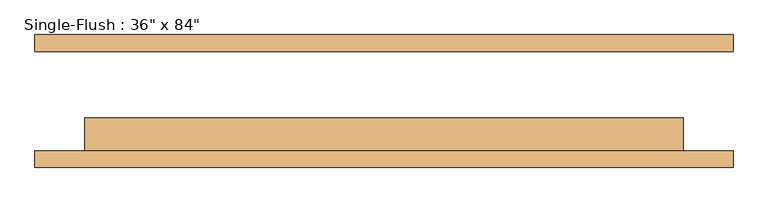
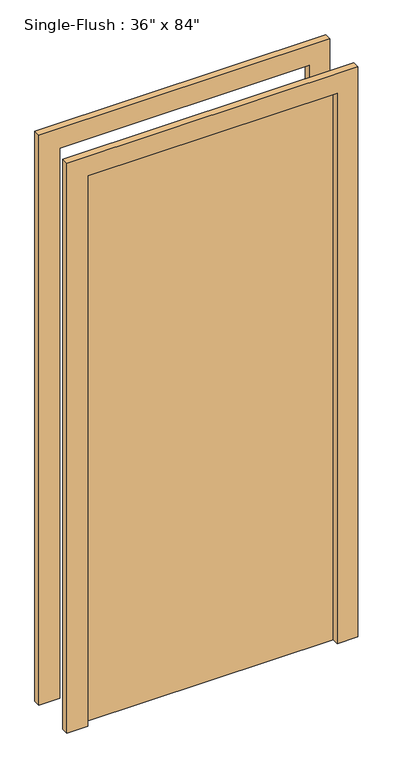
"""IFC4 building model written with IfcOpenShell, lengths in millimetres: door geometry."""

from ifc_helpers import new_model, si_unit, frame, origin, origin_with_axes, place, context, project, spatial, polyline, outline, extrude, source, transform, mapped, element, save


def door_686f89d2(model_context):
    return source(origin(), model_context, "Body", "SweptSolid", [
        extrude(outline(polyline([(2209.8, -533.4), (0.0, -533.4), (0.0, -457.2), (2133.6, -457.2), (2133.6, 457.2), (0.0, 457.2), (0.0, 533.4), (2209.8, 533.4), (2209.8, -533.4)])), frame((0.0, -101.6, 0.0), z_axis=(0.0, 1.0, 0.0), x_axis=(0.0, 0.0, 1.0)), (0.0, 0.0, 1.0), 25.4),
        extrude(outline(polyline([(2209.8, 533.4), (2209.8, -533.4), (0.0, -533.4), (0.0, -457.2), (2133.6, -457.2), (2133.6, 457.2), (0.0, 457.2), (0.0, 533.4), (2209.8, 533.4)])), frame((0.0, 76.2, 0.0), z_axis=(0.0, 1.0, 0.0), x_axis=(0.0, 0.0, 1.0)), (0.0, 0.0, 1.0), 25.4),
        extrude(outline(polyline([(457.2, -25.4), (457.2, -76.2), (-457.2, -76.2), (-457.2, -25.4), (457.2, -25.4)])), origin_with_axes(), (0.0, 0.0, 1.0), 2133.6),
    ])


if __name__ == "__main__":
    model = new_model("IFC4")
    model_context = context("Model", 3, world=origin())
    ifc_project = project(units=[si_unit("LENGTHUNIT", "METRE", prefix="MILLI")], contexts=[model_context])
    site = spatial("IfcSite", under=ifc_project)
    building = spatial("IfcBuilding", under=site)
    placement = place(None, origin())
    door_shape = door_686f89d2(model_context)
    element("IfcDoor", 1, ObjectType="Single-Flush : 36\" x 84\"", at=placement, inside=building, context=model_context, shape_type="MappedRepresentation", body=[
        mapped(door_shape, transform((0.0, 0.0, 0.0), x_axis=(1.0, 0.0, 0.0), y_axis=(0.0, 1.0, 0.0), z_axis=(0.0, 0.0, 1.0))),
    ])
    save(model, "model.ifc")

# Revit data of these elements
# Type "Single-Flush : 36\" x 84\""
#   Type Mark = "1"
#   Construction Type Id = "MDOOR"
#   Assembly Code = "C1020"
#   Analytic Construction = "Metal"
#   Thickness = 0' - 2"
#   Heat Transfer Coefficient (U) = 0.651978 BTU/(h·ft²·°F)
#   Height = 7' - 0"
#   Trim Projection Ext = 0' - 1"
#   Trim Projection Int = 0' - 1"
#   Trim Width = 0' - 3"
#   Width = 3' - 0"
#   Define Thermal Properties by = 1
#   Define Thermal Properties by = 1
#   Door Material = Door - Panel
#   Frame Material = Door - Frame
#   Visual Light Transmittance = 0
#   Solar Heat Gain Coefficient = 0
#   Function = (empty or 0)
#   Wall Closure = (empty or 0)
# Element 1 (IfcDoor, "Single-Flush : 36\" x 84\"")
#   Materials on its faces: "Door - Frame", "Door - Panel"
# Materials
#   "Door - Panel": class "Wood", colour RGB 210 159 95, transparency 0, Cost = 0
#   "Door - Frame": colour RGB 118 70 51, transparency 0, Cost = 0
